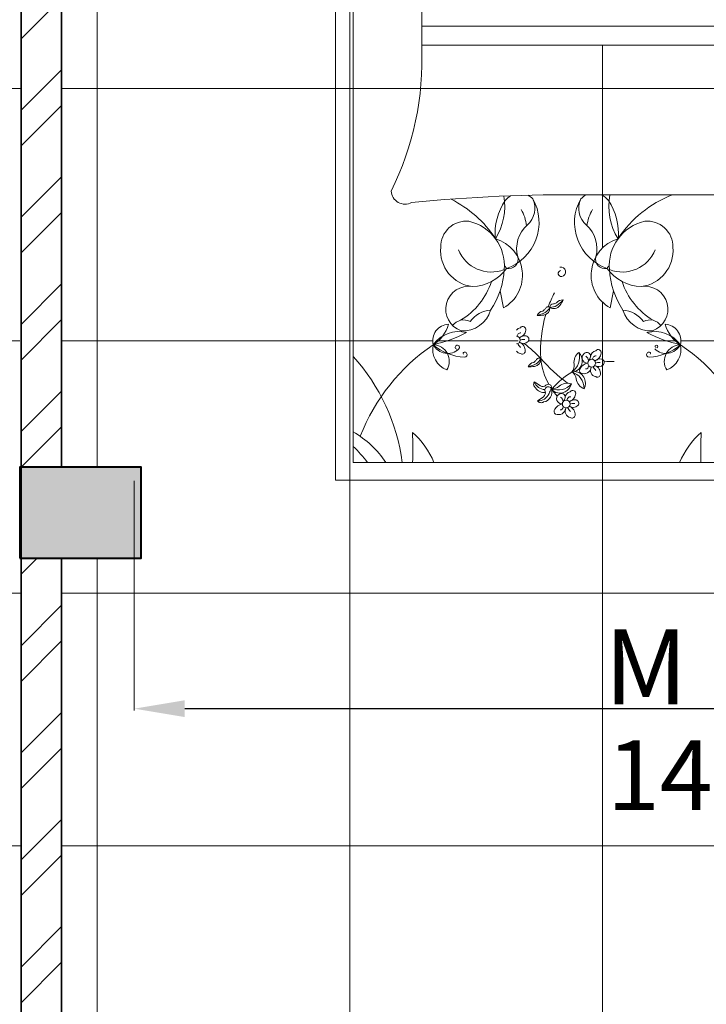
# Model space of a CAD drawing. Units: inches. Extents: x 351 to 1738, y -265 to 286.
# Tile 33 of 38: x 1380 to 1448, y 20 to 118. Entities that reach past the tile are written whole.
import ezdxf

# ---------------------------------------------------------------- set-up
doc = ezdxf.new("R2010")
doc.units = ezdxf.units.IN
doc.header["$MEASUREMENT"] = 0
for name, color, linetype, lineweight in [('A-ANNO-DIMS', 2, 'Continuous', 18), ('A-AREA-IDEN', 7, 'Continuous', 18), ('A-COLS', 7, 'Continuous', 40), ('A-COLS-PATT', 6, 'Continuous', 13), ('A-FLOR-PATT', 9, 'Continuous', 9), ('A-FURN', 18, 'Continuous', 13), ('A-WALL', 7, 'Continuous', 35), ('A-WALL-PATT', 152, 'Continuous', 13)]:
    doc.layers.add(name, color=color, linetype=linetype, lineweight=lineweight)
doc.styles.add('Annotative', font='arial.ttf')
doc.styles.get("Standard").update_dxf_attribs({"font": 'arial.ttf'})
doc.dimstyles.get("Standard").update_dxf_attribs({"dimtxt": 8, "dimasz": 5, "dimexe": 0.18, "dimexo": 0.0625, "dimgap": 0.09, "dimtad": 1, "dimtoh": 1, "dimzin": 0, "dimdsep": 46, "dimlunit": 4, "dimtxsty": 'Standard', "dimcen": 0, "dimclre": 256, "dimadec": 0, "dimazin": 0, "dimtfac": 1, "dimtofl": 0, "dimtmove": 0, "dimatfit": 3, "dimfxl": 1, "dimtolj": 1, "dimtzin": 0, "dimlwe": -1, "dimarcsym": 0})

# ---------------------------------------------------------------- blocks, each defined once
blk = doc.blocks.new('BED-DOUBLE-W-NIGHTSTANDS')
for p, q in [((121.406, 44.947), (28.441, 44.947)), ((121.549, 43.065), (28.441, 43.065)), ((106.084, 28.242), (44.816, 28.242)), ((36.536, 17.047), (36.202, 18.753)), ((47.082, 17.047), (47.416, 18.753))]:
    blk.add_line(p, q)
blk.add_lwpolyline([(28.513, 71.52, 0.001242), (28.441, 42.889, -0.127202), (25.416, 28.619)], format="xyb")
for points in [[(121.562, 54.359), (129.93, 54.359), (129.93, 0), (19.917, 0), (19.917, 54.359), (28.453, 54.359)], [(28.449, 52.61), (21.666, 52.61), (21.666, 1.749), (128.181, 1.749), (128.181, 52.61), (121.53, 52.61)]]:
    blk.add_lwpolyline(points)
for centre in [(45.254, 11.579), (42.74, 7.529)]:
    blk.add_circle(centre, 0.384)
for centre, radius, start, end in [((26.805, 28.716), 1.392, 183.97998, 297.34124), ((43.015, -128.837), 157.09, 89.34325, 95.68869), ((26.216, 17.616), 11.421, 33.66712, 63.29966), ((41.523, 24.412), 5.82, 145.78505, 184.73037), ((30.405, 27.126), 6.252, 328.82178, 9.15542), ((38.149, 26.573), 1.817, 120.0293, 142.32497), ((35.247, 25.502), 4.809, 289.28218, 29.1751), ((37.381, 26.933), 2.258, 311.56531, 23.83541), ((38.149, 26.573), 1.817, 44.45169, 63.55801), ((48.371, 25.502), 4.809, 150.8249, 250.71782), ((46.238, 26.933), 2.258, 156.16459, 228.43469), ((45.47, 26.573), 1.817, 113.22901, 135.54831), ((45.47, 26.573), 1.817, 37.67503, 66.71436), ((42.096, 24.412), 5.82, 355.26963, 34.21495), ((53.213, 27.126), 6.252, 169.71335, 211.17822), ((57.402, 17.616), 11.421, 111.49413, 146.33288), ((34.521, 24.631), 4.338, 7.43599, 29.91487), ((49.097, 24.631), 4.338, 150.08513, 172.56401), ((32.869, 23.1), 2.548, 84.48557, 181.05378), ((32.087, 21.215), 4.539, 355.29334, 76.921), ((51.531, 21.215), 4.539, 103.079, 184.70666), ((50.749, 23.1), 2.548, 358.94622, 95.51443), ((40.931, 22.929), 3.094, 131.56531, 195.14713), ((42.687, 22.929), 3.094, 344.85287, 48.43469), ((34.666, 20.299), 3.752, 299.90854, 73.1337), ((48.953, 20.299), 3.752, 106.8663, 240.09146), ((33.914, 22.735), 3.606, 174.94485, 262.88575), ((35.331, 24.102), 3.502, 201.58187, 291.42215), ((48.287, 24.102), 3.502, 248.57785, 338.41813), ((49.704, 22.735), 3.606, 277.11425, 5.05515), ((37.041, 21.876), 0.937, 257.30406, 15.14713), ((46.577, 21.876), 0.937, 164.85287, 282.69594), ((33.287, 23.537), 4.383, 272.3591, 324.04014), ((28.528, 21.336), 8.098, 326.28828, 356.5076), ((41.523, 24.412), 5.82, 212.70113, 216.34448), ((42.242, 20.456), 0.291, 102.70507, 280.43845), ((42.209, 20.635), 0.473, 280.43845, 100.41356), ((42.096, 24.412), 5.82, 323.65552, 327.29887), ((50.331, 23.537), 4.383, 215.95986, 267.6409), ((55.091, 21.336), 8.098, 183.4924, 213.71172), ((28.594, 21.91), 7.124, 301.26137, 341.7045), ((55.024, 21.91), 7.124, 198.2955, 238.73863), ((33.085, 16.925), 2.265, 80.26398, 250.86884), ((52.702, 12.86), 12.498, 153.0032, 159.89408), ((50.534, 16.925), 2.265, 289.13116, 99.73602), ((40.818, 19.778), 2.424, 285.51291, 293.60991), ((42.4, 17.052), 0.792, 87.35788, 140.49441), ((40.569, 19.327), 2.385, 301.16403, 321.56124), ((38.629, 19.743), 4.256, 324.68979, 333.49364), ((32.541, 17.606), 2.828, 265.96902, 344.3045), ((35.587, 13.847), 3.012, 96.1662, 141.58255), ((40.576, 15.96), 0.792, 101.32561, 154.46214), ((39.436, 18.648), 2.385, 280.25878, 300.65599), ((38.921, 18.642), 2.424, 308.21012, 316.30712), ((40.408, 17.049), 0.724, 278.34322, 4.28685), ((40.007, 17.685), 1.265, 300.65599, 332.63414), ((40.958, 16.849), 0.307, 55.76575, 157.44165), ((41.436, 17.136), 0.307, 84.37838, 186.05427), ((41.149, 18.368), 1.265, 269.18588, 301.16403), ((41.519, 17.714), 0.724, 237.53317, 323.47681), ((48.031, 13.847), 3.012, 38.41745, 83.8338), ((51.077, 17.606), 2.828, 195.6955, 274.03098), ((32.618, 14.471), 1.388, 63.97555, 143.26805), ((39.985, 20.555), 4.256, 268.32639, 277.13024), ((52.702, 12.86), 12.498, 163.58418, 183.82768), ((51, 14.471), 1.388, 36.73195, 116.02445), ((31.166, 13.794), 1.634, 92.95159, 193.72796), ((27.826, 16.28), 3.366, 301.38267, 345.29688), ((32.107, 11.586), 3.115, 75.46535, 144.23429), ((38.336, 14.458), 0.641, 101.56373, 142.6358), ((37.821, 14.961), 0.924, 288.72627, 352.50315), ((38.45, 14.916), 0.297, 345.23556, 144.9248), ((51.511, 11.586), 3.115, 35.76571, 104.53465), ((52.452, 13.794), 1.634, 346.27204, 87.04841), ((55.792, 16.28), 3.366, 194.70312, 238.61733), ((26.591, 26.864), 13.785, 282.51726, 297.18239), ((37.804, 13.863), 0.384, 273.27684, 86.72316), ((38.252, 14.227), 0.367, 91.10805, 181.86747), ((38.642, 13.489), 0.794, 80.3487, 133.65382), ((38.499, 14.146), 0.629, 229.78892, 317.67915), ((38.491, 12.663), 1.258, 83.08516, 105.71709), ((38.719, 13.945), 0.331, 317.67915, 80.3487), ((57.027, 26.864), 13.785, 242.81761, 257.48274), ((40.708, -2.855), 19.706, 124.38655, 158.59079), ((31.714, 12.942), 2.185, 167.71153, 249.03868), ((29.53, 11.762), 1.646, 328.46331, 88.28689), ((32.859, 17.159), 4.984, 228.84017, 267.9352), ((31.007, 14.156), 1.612, 207.6827, 313.77619), ((31.974, 13.146), 0.213, 313.77619, 249.71835), ((38.328, 13.152), 0.634, 217.76209, 259.04026), ((39.013, 13.997), 1.167, 203.42757, 227.61037), ((37.791, 12.814), 0.893, 355.05304, 68.36176), ((38.387, 12.763), 0.295, 232.47371, 355.05304), ((29.779, 2.226), 14.328, 43.15413, 52.0459), ((45.785, 12.175), 0.641, 101.56373, 176.36503), ((45.9, 12.632), 0.297, 345.23556, 144.9248), ((50.759, 17.159), 4.984, 272.0648, 311.15983), ((52.612, 14.156), 1.612, 226.22381, 332.3173), ((51.667, 13.227), 0.128, 290.26671, 226.22708), ((54.088, 11.762), 1.646, 91.71311, 211.53669), ((51.904, 12.942), 2.185, 290.96132, 12.28847), ((42.91, -2.855), 19.706, 21.40921, 55.61345), ((6.995, -0.907), 19.706, 7.74496, 41.8856), ((32.663, 12.546), 0.119, 101.4834, 217.94089), ((32.688, 12.423), 0.245, 267.9352, 101.4834), ((38.022, 13.564), 2.424, 308.21012, 316.30712), ((39.509, 11.972), 0.724, 278.34322, 4.28685), ((39.108, 12.607), 1.265, 300.65599, 332.63414), ((40.059, 11.772), 0.307, 55.76575, 157.44165), ((46.476, 12.545), 6.266, 184.75602, 209.20408), ((55.496, 25.887), 20.619, 222.24124, 232.17444), ((42.312, 12.15), 1.752, 304.53686, 16.36991), ((44.744, 11.659), 1.239, 127.31045, 187.92519), ((43.042, 11.798), 1.273, 355.01064, 41.65801), ((44.83, 12.114), 0.524, 126.10456, 271.42811), ((44.771, 12.256), 0.377, 353.75256, 131.70535), ((44.417, 11.809), 0.529, 0.06451, 61.15075), ((44.543, 12.26), 0.604, 311.84125, 355.78771), ((45.702, 11.943), 0.367, 91.10805, 181.86747), ((46.092, 11.205), 0.794, 80.3487, 133.65382), ((45.271, 12.677), 0.924, 288.72627, 352.50315), ((46.169, 11.661), 0.331, 317.67915, 80.3487), ((47.12, 4.223), 7.516, 87.10709, 94.75853), ((50.93, 12.423), 0.245, 78.5166, 272.0648), ((50.955, 12.546), 0.119, 322.05911, 78.5166), ((39.677, 10.882), 0.792, 101.32561, 154.46214), ((38.537, 13.571), 2.385, 280.25878, 300.65599), ((39.086, 15.478), 4.256, 268.32639, 277.13024), ((43.248, 11.759), 1.065, 272.84988, 356.12261), ((42.496, 11.346), 1.031, 321.76073, 7.92519), ((43.551, 9.683), 1.065, 20.5253, 88.5375), ((44.446, 10.858), 0.381, 148.0499, 225.62681), ((47.12, 4.223), 7.516, 113.05007, 113.84774), ((45.151, 10.418), 1.212, 104.75581, 148.0499), ((44.472, 11.286), 0.758, 247.40857, 351.43859), ((44.685, 11.255), 0.255, 262.90601, 7.13198), ((45.778, 10.868), 0.634, 151.21959, 259.04026), ((46.463, 11.713), 1.167, 203.42757, 227.61037), ((45.949, 11.862), 0.629, 229.78892, 317.67915), ((45.241, 10.53), 0.893, 355.05304, 68.36176), ((45.941, 10.379), 1.258, 83.08516, 105.71709), ((47.12, 4.223), 7.516, 120.54402, 139.81798), ((42.712, 9.864), 1.031, 8.72271, 54.88717), ((42.767, 9.04), 1.752, 0.278, 72.11105), ((44.956, 10.208), 1.239, 188.72271, 249.33746), ((43.365, 9.587), 1.273, 334.9899, 21.63727), ((45.837, 10.479), 0.295, 232.47371, 355.05304), ((39.944, 9.493), 0.429, 146.86359, 236.90213), ((45.994, 18.945), 11.227, 235.1882, 238.88441), ((40.68, 10.115), 1.162, 199.47987, 267.68284), ((40.551, 9.675), 1, 212.81548, 277.39917), ((40.422, 9.714), 0.444, 238.88441, 314.26458), ((40.325, 8.719), 1, 280.30568, 17.1958), ((40.241, 8.615), 0.444, 306.37461, 21.75478), ((40.965, 8.904), 0.335, 19.36054, 201.75478), ((40.966, 9.155), 0.335, 311.87034, 134.26458), ((47.267, 6.101), 6.693, 153.78194, 158.29129), ((41.94, 10.674), 1.752, 247.23048, 319.06353), ((41.362, 10.084), 1.031, 264.45436, 310.61881), ((46.476, 12.545), 6.266, 214.00334, 222.49171), ((42.116, 9.675), 1.065, 218.32082, 298.81623), ((42.84, 8.361), 1.239, 70.00407, 130.61881), ((42.038, 9.869), 1.273, 297.70426, 344.35163), ((43.386, 8.581), 0.297, 345.23556, 144.9248), ((39.969, 9.007), 1.162, 266.97007, 338.29129), ((33.846, 17.297), 11.227, 302.6784, 306.37461), ((40.262, 8.089), 0.429, 214.3538, 304.39233), ((42.316, 8.063), 0.524, 126.10456, 271.42811), ((42.258, 8.205), 0.377, 353.75256, 131.70535), ((41.904, 7.758), 0.529, 0.06451, 61.15075), ((42.029, 8.209), 0.604, 311.84125, 355.78771), ((43.272, 8.124), 0.641, 101.56373, 176.36503), ((43.188, 7.892), 0.367, 91.10805, 181.86747), ((43.578, 7.154), 0.794, 80.3487, 133.65382), ((42.757, 8.626), 0.924, 288.72627, 352.50315), ((43.656, 7.611), 0.331, 317.67915, 80.3487), ((41.933, 6.807), 0.381, 148.0499, 225.62681), ((42.638, 6.368), 1.212, 104.75581, 148.0499), ((41.958, 7.235), 0.758, 247.40857, 351.43859), ((42.171, 7.205), 0.255, 262.90601, 7.13198), ((43.264, 6.817), 0.634, 151.21959, 259.04026), ((43.949, 7.662), 1.167, 203.42757, 227.61037), ((43.436, 7.811), 0.629, 229.78892, 317.67915), ((42.727, 6.48), 0.893, 355.05304, 68.36176), ((43.427, 6.328), 1.258, 83.08516, 105.71709), ((43.323, 6.428), 0.295, 232.47371, 355.05304), ((16.881, -3.546), 9.602, 33.46172, 60.11157), ((22.259, -1.325), 8.012, 22.55474, 48.95456), ((0.311, 2.982), 27.264, 357.40811, 3.65191), ((61.36, -1.325), 8.012, 131.04544, 157.44526), ((83.307, 2.982), 27.264, 176.34809, 182.59189), ((13.426, -5.336), 11.966, 36.30357, 46.48142)]:
    blk.add_arc(centre, radius, start, end)
blk = doc.blocks.new('COL-9x12')
blk.add_lwpolyline([(0, 12), (0, 0), (9, 0), (9, 12)], close=True)
blk = doc.blocks.new('*D46')
at = {"layer": 'A-ANNO-DIMS', "transparency": 16777216}
for p, q in [((1391.393, 72.125), (1391.393, 49.373)), ((1542.294, 72.125), (1542.294, 49.373))]:
    blk.add_line(p, q, dxfattribs=at)
at = {"layer": 'A-ANNO-DIMS', "color": 0, "lineweight": -2, "transparency": 16777216}
for p, q in [((1396.393, 49.553), (1537.294, 49.553)), ((1542.294, 49.553), (1738.088, 49.553))]:
    blk.add_line(p, q, dxfattribs=at)
at = {"layer": 'A-ANNO-DIMS', "color": 0, "transparency": 16777216}
for points in [[(1396.393, 50.386), (1396.393, 48.72), (1391.393, 49.553)], [(1537.294, 50.386), (1537.294, 48.72), (1542.294, 49.553)]]:
    blk.add_solid(points, dxfattribs=at)
at = {"layer": 'Defpoints', "color": 0, "transparency": 16777216}
for p in [(1391.393, 72.188), (1542.294, 72.188), (1542.294, 49.553)]:
    blk.add_point(p, dxfattribs=at)
at = {"layer": 'A-ANNO-DIMS', "color": 0, "transparency": 16777216, "insert": (1642.691, 53.779), "char_height": 8, "attachment_point": 5}
blk.add_mtext('\\A1;BED AND NIGHTSTANDS 12\'-7" TYP.', dxfattribs=at)

msp = doc.modelspace()

# ---------------------------------------------------------------- hatches: boundary and pattern name
at = {"layer": 'A-COLS-PATT'}
h = msp.add_hatch(color=256, dxfattribs=at)
h.dxf.hatch_style = 1
h.paths.add_polyline_path([(1112.704, 237.963), (1103.704, 237.963), (1103.704, 228.963), (1112.704, 228.963)])
h.paths.add_polyline_path([(1115.704, 237.963), (1112.704, 237.963), (1112.704, 228.963), (1115.704, 228.963)])
h.paths.add_polyline_path([(1043.704, 255.963), (1034.704, 255.963), (1034.704, 243.963), (1043.704, 243.963)])
h.paths.add_polyline_path([(1043.704, 210.963), (1034.704, 210.963), (1034.704, 198.963), (1043.704, 198.963)])
h.paths.add_polyline_path([(1043.704, -45.037), (1034.704, -45.037), (1034.704, -57.037), (1043.704, -57.037)])
h.paths.add_polyline_path([(1112.704, -45.037), (1103.704, -45.037), (1103.704, -57.037), (1112.704, -57.037)])
h.paths.add_polyline_path([(1112.704, -161.037), (1103.704, -161.037), (1103.704, -164.037), (1103.704, -173.037), (1112.704, -173.037)])
h.paths.add_polyline_path([(1043.704, -161.037), (1034.704, -161.037), (1034.704, -173.037), (1043.704, -173.037)])
h.paths.add_polyline_path([(1248.549, -164.037), (1236.549, -164.037), (1236.549, -173.037), (1248.549, -173.037)])
h.paths.add_polyline_path([(1248.549, -50), (1236.549, -50), (1236.549, -59), (1248.549, -59)])
h.paths.add_polyline_path([(1248.704, 73.463), (1244.704, 73.463), (1244.704, 64.463), (1248.704, 64.463)])
h.paths.add_polyline_path([(1244.704, 73.463), (1236.704, 73.463), (1236.704, 64.463), (1244.704, 64.463)])
h.paths.add_polyline_path([(1248.704, 237.963), (1236.704, 237.963), (1236.704, 228.963), (1248.704, 228.963)])
h.paths.add_polyline_path([(1392.204, 237.963), (1380.204, 237.963), (1380.204, 228.963), (1392.204, 228.963)])
h.paths.add_polyline_path([(1536.064, 237.963), (1524.064, 237.963), (1524.064, 228.963), (1536.064, 228.963)])
h.paths.add_polyline_path([(1536.064, 73.463), (1524.064, 73.463), (1524.064, 64.463), (1536.064, 64.463)])
h.paths.add_polyline_path([(1384.204, 73.463), (1380.204, 73.463), (1380.204, 64.463), (1384.204, 64.463)])
h.paths.add_polyline_path([(1392.064, 73.463), (1384.204, 73.463), (1384.204, 64.463), (1392.064, 64.463)])
h.paths.add_polyline_path([(1536.064, -53.037), (1524.064, -53.037), (1524.064, -57.037), (1536.064, -57.037)])
h.paths.add_polyline_path([(1536.064, -48.037), (1524.064, -48.037), (1524.064, -53.037), (1536.064, -53.037)])
h.paths.add_polyline_path([(1392.064, -48.037), (1380.064, -48.037), (1380.064, -56.5), (1380.065, -57.037), (1392.064, -57.037)])
h.paths.add_polyline_path([(1536.064, -164.037), (1524.064, -164.037), (1524.064, -173.037), (1536.064, -173.037)])
at = {"layer": 'A-FLOR-PATT', "transparency": 33554559}
h = msp.add_hatch(dxfattribs=at)
h.set_pattern_fill('ANSI37', color=256, scale=200, angle=135)
h.set_pattern_definition([(180, (1112.704, -164.037), (-2e-15, -25), []), (270, (1112.704, -164.037), (25, -5e-15), [])])
h.paths.add_polyline_path([(1380.064, 73.463), (1380.132, 148.463), (1338.064, 148.463), (1290.704, 148.463), (1290.704, 88.463), (1248.704, 88.463), (1248.704, -2.009), (1244.704, -2.009), (1244.704, 142.457), (1160.704, 142.457), (1160.704, 158.963), (1160.704, 170.137), (1160.704, 206.137), (1160.704, 228.963), (1112.704, 228.963), (1112.704, 209.963), (1112.704, 168.963), (1124.704, 168.963), (1124.704, 162.963), (1112.704, 162.963), (1112.704, 64.463), (1112.704, 60.463), (1112.704, 0.463), (1112.704, -48.026), (1146.804, -47.981), (1146.804, -35.691), (1207.804, -35.691), (1207.804, -47.902), (1236.542, -47.864), (1236.544, -50.009), (1248.5, -50.009), (1248.506, -102.915), (1248.512, -150.915), (1248.514, -164.037), (1248.549, -164.037), (1273.017, -164.037), (1273.017, -128.799), (1355.24, -128.799), (1355.24, -164.037), (1384.204, -164.037), (1384.204, -57.037), (1380.064, -57.037), (1380.064, -48.037), (1392.064, -48.037), (1392.064, -53.037), (1406.549, -53.037), (1406.549, -57.037), (1401.204, -57.037), (1401.204, -147.037), (1468.204, -147.037), (1468.204, -138.5), (1472.204, -138.5), (1472.204, -102.5), (1468.204, -102.5), (1468.204, -57.037), (1442.549, -57.037), (1442.549, -53.037), (1463.049, -53.037), (1463.049, -40.747), (1524.049, -40.747), (1524.049, -48.037), (1536.064, -48.037), (1536.064, -53.037), (1557.704, -53.037), (1557.704, 204.963), (1384.204, 204.963), (1384.204, 73.463), (1392.064, 73.463), (1392.064, 64.463), (1384.204, 64.463), (1384.204, -3.5), (1380.204, -3.537), (1380.204, 64.463), (1380.064, 64.463)])
h.paths.add_polyline_path([(1510.714, 86.458, -0.103984), (1511.661, 85.595, 0.470438), (1510.158, 87.614, 0.0961)], flags=16)
h.paths.add_polyline_path([(1510.443, 100.266, 0.009798), (1504.693, 100.48, 0.02879), (1504.6, 99.767, -0.165331), (1505.519, 96.135, -0.143601)], flags=16)
h.paths.add_polyline_path([(1487.201, 85.595, -0.103984), (1488.148, 86.458, 0.0961), (1488.704, 87.614, 0.470438)], flags=0)
h.paths.add_polyline_path([(1495.052, 100.43), (1494.178, 100.43, -0.026463), (1494.262, 99.774, -0.144219)], flags=16)
h.paths.add_polyline_path([(1444.485, 86.458, -0.103984), (1445.433, 85.595, 0.470438), (1443.93, 87.614, 0.0961)], flags=16)
h.paths.add_polyline_path([(1420.972, 85.595, -0.103984), (1421.92, 86.458, 0.0961), (1422.475, 87.614, 0.470438)], flags=16)
h.paths.add_polyline_path([(1428.632, 100.335, 0.001054), (1427.971, 100.309, -0.021524), (1428.033, 99.774, -0.114301)], flags=16)
h.paths.add_polyline_path([(1419.906, 143.708, 0.024979), (1420.222, 157.526), (1421.573, 159.101), (1421.573, 175.369), (1391.393, 175.369), (1391.393, 200.519), (1542.294, 200.519), (1542.294, 175.369), (1512.028, 175.369, 0.019865), (1511.521, 153.838, 0.025134), (1512.758, 118.323, 0.020553), (1512.942, 115.253), (1419.834, 115.253, -0.000414), (1419.843, 124.798), (1413.059, 124.798), (1413.059, 84.437, -0.061853), (1415.831, 80.45, -0.093077), (1420.972, 85.595, -0.267537), (1422.371, 84.732, 0.08511), (1424.052, 84.616, -0.885393), (1424.033, 84.851, -1.125815), (1424.073, 84.366, -0.087987), (1422.371, 84.732, -0.267537), (1422.326, 83.089, -0.370542), (1420.972, 85.595, 0.093077), (1415.831, 80.45, -0.087414), (1417.914, 73.937), (1418.941, 73.937, 0.02725), (1418.913, 76.906, -0.115703), (1421.051, 73.937), (1445.354, 73.937, -0.115703), (1447.492, 76.906, 0.02725), (1447.464, 73.937), (1448.491, 73.937, -0.087414), (1450.574, 80.45, 0.093077), (1445.433, 85.595, -0.370542), (1444.079, 83.089, -0.267537), (1444.034, 84.732, -0.087987), (1442.332, 84.366, -1.125815), (1442.372, 84.851, -2.032736), (1442.364, 84.368, 0.086378), (1444.034, 84.732, -0.267537), (1445.433, 85.595, -0.093077), (1450.574, 80.45, -0.257732), (1466.483, 90.927, -0.47867), (1468.832, 91.907, -0.47867), (1471.18, 90.927, -0.26264), (1483.053, 81.78, -0.071866), (1487.201, 85.595, -0.267537), (1488.6, 84.732, 0.08511), (1490.28, 84.616, -0.885393), (1490.262, 84.851, -1.125815), (1490.301, 84.366, -0.087987), (1488.6, 84.732, -0.267537), (1488.554, 83.089, -0.370542), (1487.201, 85.595, 0.071866), (1483.053, 81.78, -0.132065), (1484.143, 73.937), (1485.169, 73.937, 0.02725), (1485.142, 76.906, -0.115703), (1487.28, 73.937), (1511.582, 73.937, -0.115703), (1513.72, 76.906, 0.02725), (1513.693, 73.937), (1514.719, 73.937, -0.087414), (1516.802, 80.45, 0.093077), (1511.661, 85.595, -0.370542), (1510.308, 83.089, -0.267537), (1510.262, 84.732, -0.087987), (1508.561, 84.366, -1.125815), (1508.601, 84.851, -2.032736), (1508.592, 84.368, 0.086378), (1510.262, 84.732, -0.267537), (1511.661, 85.595, -0.093077), (1516.802, 80.45, -0.061853), (1519.575, 84.437), (1519.575, 73.937), (1413.059, 73.937), (1413.059, 124.798), (1419.843, 124.798, -0.000821)], flags=16)
h.paths.add_polyline_path([(1220.149, 54.133, -0.103984), (1220.869, 53.476, 0.470438), (1219.727, 55.011, 0.0961)], flags=16)
h.paths.add_polyline_path([(1219.944, 64.626, 0.009798), (1215.574, 64.789, 0.02879), (1215.503, 64.247, -0.165331), (1216.201, 61.487, -0.143601)], flags=16)
h.paths.add_polyline_path([(1209.779, 64.449, 0.097446), (1209.339, 64.751), (1208.247, 64.751, 0.12739), (1207.7, 64.326, 0.171586), (1206.95, 61.475, -0.158854), (1207.636, 59.45, 0.015898), (1207.795, 59.218, 0.061546), (1208.598, 59.616, 0.175416), (1208.638, 60.099, -0.284779), (1209.348, 62.472, 0.326216)], flags=16)
h.paths.add_polyline_path([(1169.818, 54.133, -0.103984), (1170.538, 53.476, 0.470438), (1169.396, 55.011, 0.0961)], flags=16)
h.paths.add_polyline_path([(1159.017, 62.472, 0.284764), (1158.307, 60.099, -0.175433), (1158.267, 59.616, 0.39293), (1159.448, 64.449, -0.32623)], flags=16)
h.paths.add_polyline_path([(1156.342, 58.239, -0.178321), (1154.011, 55.31, -0.174736), (1154.722, 55.233, -0.200802), (1156.27, 56.086, 0.12699), (1157.283, 58.991, -0.091205)], flags=16)
h.paths.add_polyline_path([(1156.624, 61.413, 0.157275), (1157.316, 64.247, 0.169622)], flags=16)
h.paths.add_polyline_path([(1152.67, 54.133, -0.0961), (1151.95, 53.476, 0.064076), (1154.465, 54.384, 0.199016)], flags=16)
h.paths.add_polyline_path([(1202.281, 53.476, -0.103984), (1203, 54.133, 0.0961), (1203.423, 55.011, 0.470438)], flags=0)
h.paths.add_polyline_path([(1151.139, 97.64, 0.024979), (1151.379, 108.141), (1152.406, 109.338), (1152.406, 121.701), (1129.47, 121.701), (1129.47, 140.814), (1244.149, 140.814), (1244.149, 121.701), (1221.148, 121.701, 0.019865), (1220.763, 105.338, 0.025134), (1221.703, 78.349, 0.020553), (1221.843, 76.016), (1151.078, 76.016, -0.128743), (1148.786, 65.037, 0.539352), (1150.327, 64.171, -0.027594), (1163.481, 64.751, 0.097695), (1163.04, 64.449, 0.326216), (1163.471, 62.472, -0.284777), (1164.181, 60.099, -0.194757), (1165.846, 61.443, -0.155402), (1165.172, 64.247, -0.166022), (1165.869, 61.475, -0.177014), (1167.852, 62.77, -0.448203), (1169.974, 60.807, -0.393499), (1167.679, 57.86, -0.895548), (1168.438, 54.524, -0.355767), (1166.218, 56.086, -0.066024), (1165.505, 57.539), (1165.251, 56.243, -0.371732), (1164.02, 59.758, -0.373614), (1163.04, 64.449, -0.097695), (1163.481, 64.751, 0.021354), (1153.294, 64.429, -0.134183), (1156.695, 61.368, 0.186873), (1154.636, 62.77, 0.448203), (1152.514, 60.807, 0.403726), (1154.905, 57.846, 0.711219), (1153.334, 55, 0.53154), (1151.95, 53.476, -0.267537), (1153.013, 52.821, 0.08511), (1154.29, 52.732, -0.885393), (1154.276, 52.911, -1.125815), (1154.306, 52.543, -0.087987), (1153.013, 52.821, -0.267537), (1152.978, 51.572, -0.370542), (1151.95, 53.476, 0.093077), (1148.043, 49.566, -0.087414), (1149.626, 44.617), (1150.406, 44.617, 0.02725), (1150.385, 46.873, -0.115703), (1152.01, 44.617), (1170.478, 44.617, -0.115703), (1172.103, 46.873, 0.02725), (1172.082, 44.617), (1172.862, 44.617, -0.087414), (1174.445, 49.566, 0.093077), (1170.538, 53.476, -0.370542), (1169.51, 51.572, -0.267537), (1169.475, 52.821, -0.087987), (1168.182, 52.543, -1.125815), (1168.212, 52.911, -2.032736), (1168.206, 52.544, 0.086378), (1169.475, 52.821, -0.267537), (1170.538, 53.476, -0.093077), (1174.445, 49.566, -0.257732), (1186.536, 57.528, -0.47867), (1188.321, 58.273, -0.47867), (1190.106, 57.528, -0.26264), (1199.128, 50.577, -0.071866), (1202.281, 53.476, -0.267537), (1203.344, 52.821, 0.08511), (1204.621, 52.732, -0.885393), (1204.607, 52.911, -1.125815), (1204.637, 52.543, -0.087987), (1203.344, 52.821, -0.267537), (1203.309, 51.572, -0.370542), (1202.281, 53.476, 0.071866), (1199.128, 50.577, -0.132065), (1199.957, 44.617), (1200.737, 44.617, 0.02725), (1200.716, 46.873, -0.115703), (1202.341, 44.617), (1220.809, 44.617, -0.115703), (1222.434, 46.873, 0.02725), (1222.413, 44.617), (1223.193, 44.617, -0.087414), (1224.776, 49.566, 0.093077), (1220.869, 53.476, -0.370542), (1219.841, 51.572, -0.267537), (1219.806, 52.821, -0.087987), (1218.513, 52.543, -1.125815), (1218.543, 52.911, -2.032736), (1218.537, 52.544, 0.086378), (1219.806, 52.821, -0.267537), (1220.869, 53.476, -0.093077), (1224.776, 49.566, -0.061853), (1226.883, 52.597), (1226.883, 44.617), (1145.936, 44.617), (1145.936, 83.269), (1151.091, 83.269, -0.000821)], flags=16)
h.paths.add_polyline_path([(1218.01, 57.86, -0.895548), (1218.769, 54.524, -0.355767), (1216.549, 56.086, -0.066024), (1215.836, 57.539), (1215.582, 56.243, -0.371732), (1214.351, 59.758, -0.373614), (1213.371, 64.449, 0.326216), (1213.802, 62.472, -0.284777), (1214.512, 60.099, -0.194757), (1216.177, 61.443, -0.179991), (1218.183, 62.77, -0.448203), (1220.305, 60.807, -0.393499)], flags=16)
h.paths.add_polyline_path([(1424.735, 91.363, -0.393499), (1421.715, 95.241, -0.448203), (1424.507, 97.824, -0.179991), (1427.147, 96.077, -0.194757), (1429.338, 94.309, -0.284777), (1430.272, 97.432, 0.326216), (1430.839, 100.034, -0.373614), (1429.55, 93.861, -0.371732), (1427.929, 89.235), (1427.596, 90.941, -0.066024), (1426.657, 89.029, -0.355767), (1423.736, 86.973, -0.895548)], flags=16)
h.paths.add_polyline_path([(1238.033, 131.257, -1), (1227.329, 131.257, -1)], flags=0)
h.paths.add_polyline_path([(1235.357, 131.257, -1), (1230.005, 131.257, -1)], flags=0)
h.paths.add_polyline_path([(1214.039, 54.243, 0.154382), (1214.38, 53.992, 0.358955), (1213.613, 54.016, 0.603948), (1214.379, 53.657, 0.371319), (1213.968, 52.872, 0.187994), (1214.312, 52.809, -0.592455), (1213.953, 52.967, -0.294279), (1214.083, 53.691, -1.300187), (1213.881, 54.134, -0.283762), (1214.469, 53.896, 1.15094)], flags=16)
h.paths.add_polyline_path([(1212.091, 56.286, -0.408434), (1211.337, 56.445, -0.036259), (1211.098, 56.848, -0.236098), (1211.59, 56.63, 0.035345), (1211.835, 56.543, -0.475241), (1212.091, 56.286, -0.475241), (1212.438, 56.182, 0.035345), (1212.631, 56.007, -0.236098), (1213.056, 55.676, -0.036259), (1212.588, 55.697, -0.408434)], flags=16)
h.paths.add_polyline_path([(1211.469, 50.297, 0.296043), (1210.47, 50.527, 0.310883), (1211.931, 50.148, 0.021255)], flags=16)
h.paths.add_polyline_path([(1213.739, 51.818, -0.036259), (1213.271, 51.838, -0.408434), (1212.774, 52.427, -0.094786), (1212.293, 50.703, 1.150474), (1212.911, 50.232, 0.166288), (1213.265, 50.68, -0.025254), (1212.603, 50.13, 1.087932), (1212.471, 49.407, 0.166288), (1213.02, 49.251, -0.016128), (1212.567, 49.563, -0.286859), (1212.217, 49.638, 0.022156), (1212.046, 50.055, -0.64613), (1212.185, 50.498, 0.088412), (1212.732, 52.077, -1.186037), (1213.121, 52.323, 0.035345), (1213.314, 52.148, -0.236098)], flags=16)
h.paths.add_polyline_path([(1212.094, 50.342, -0.048524), (1211.54, 49.605, -1.103834), (1211.397, 48.738, -0.785515), (1211.683, 48.254, -0.392043), (1210.948, 48.525, -0.392819), (1210.561, 47.995, -0.592455), (1210.201, 48.153, -0.294279), (1210.331, 48.877, -0.704172), (1210.316, 49.592, -0.679344), (1210.729, 50.112, 0.563676)], flags=16)
h.paths.add_polyline_path([(1211.274, 49.829, -0.139826), (1210.745, 49.859, -0.217879), (1210.948, 49.509, -0.498572)], flags=0)
h.paths.add_polyline_path([(1433.426, 81.49, -0.181571), (1434.245, 81.788, -0.008067), (1433.726, 82.205, 0.045578), (1432.755, 81.242, 0.179011)], flags=16)
h.paths.add_polyline_path([(1434.146, 81.009, -0.132442), (1433.645, 80.771, 0.259089), (1433.234, 80.471, -0.180211), (1433.392, 80.805, -0.16994), (1432.758, 81.109, 0.032652), (1433.273, 80.474, -0.493363), (1434.046, 80.146, -0.390497)], flags=16)
h.paths.add_polyline_path([(1434.83, 80.047, -0.947538), (1435.294, 79.576, -0.299128), (1434.625, 79.404, -0.270439), (1435.01, 78.591, -0.592455), (1434.537, 78.382, -0.392819), (1434.027, 79.08, -0.392043), (1433.06, 78.723, -0.352042), (1433.003, 79.197, -0.197216), (1433.75, 79.734, -0.71364), (1434.447, 79.939, -0.21479), (1434.819, 80.475, 0.408833), (1435.075, 80.803, -0.226152)], flags=16)
h.paths.add_polyline_path([(1432.67, 81.217, -0.454218), (1431.897, 79.923, -0.414411), (1431.301, 80.035, 0.016129), (1431.897, 80.445, 0.27957), (1432.073, 80.871, -0.289504), (1431.103, 81.321, -0.414411), (1430.978, 81.915, 0.01613), (1431.586, 81.521, 0.341293), (1432.125, 81.583, -0.813186)], flags=16)
h.paths.add_polyline_path([(1429.893, 86.381, -0.947538), (1430.358, 85.91, -0.173106), (1429.984, 85.712, -0.038817), (1431.625, 84.214, -0.0879), (1432.097, 88.549, -0.049768), (1431.254, 88.49, -0.236098), (1431.814, 88.925, 0.035345), (1432.067, 89.155, -0.475241), (1432.524, 89.291, -0.475241), (1432.86, 89.63, 0.035345), (1433.182, 89.744, -0.236098), (1433.83, 90.032, -0.036259), (1433.516, 89.502, -0.408434), (1432.524, 89.291, -0.312424), (1432.106, 88.58, 0.088559), (1431.625, 84.214, -0.408434), (1430.971, 83.439, -0.036259), (1430.355, 83.412, -0.236098), (1430.914, 83.847, 0.035345), (1431.168, 84.078, -0.475241), (1431.625, 84.214, 0.038817), (1429.984, 85.712, -0.321732), (1429.333, 86.048, -0.32743), (1429.883, 86.809, 0.408833), (1430.138, 87.138, -0.226152)], flags=16)
h.paths.add_polyline_path([(1211.206, 58.616, -0.999784), (1211.336, 59.323, -0.614994)], flags=16)
h.paths.add_polyline_path([(1210.288, 49.429, 0.154382), (1210.629, 49.178, 0.358955), (1209.861, 49.202, 0.603948), (1210.627, 48.843, -0.534825), (1210.806, 49.295, 0.748346)], flags=16)
h.paths.add_polyline_path([(1209.589, 51.828, -0.008791), (1209.775, 51.753, 0.112231), (1209.466, 52.019, 1.418851), (1209.014, 51.708, -0.458726), (1208.651, 51.073, -0.592455), (1208.291, 51.232, -0.294279), (1208.421, 51.955, -1.300187), (1208.219, 52.398, -0.226005), (1208.719, 52.257, -0.475519), (1209.158, 52.369, -1.455499), (1209.603, 52.664, 0.421305), (1209.191, 52.262, -0.591212), (1208.979, 51.796, 0.497399), (1209.773, 51.333, 0.649312)], flags=16)
h.paths.add_polyline_path([(1208.029, 52.041, 0.544667), (1208.832, 52.045, 0.220132)], flags=0)
h.paths.add_polyline_path([(1210.438, 51.425, -0.2042), (1210.277, 52.018, 0.270826), (1209.915, 52.897, 0.324115)], flags=0)
h.paths.add_polyline_path([(1209.668, 52.407, -0.60139), (1208.99, 52.221, -0.394916), (1208.248, 52.83, -0.836792), (1208.651, 53.017, -0.338488), (1209.039, 52.571, 0.194138), (1209.191, 52.262, 0.413995), (1209.712, 52.475, 0.51771), (1210.503, 51.416, 0.401922), (1209.493, 50.93, 0.206396), (1209.516, 50.165, -0.319463), (1210.417, 51.418, -0.466635)], flags=16)
h.paths.add_polyline_path([(1206.601, 56.086, -0.355767), (1204.381, 54.524, -0.921198), (1205.236, 57.846, 0.206569), (1207.614, 58.991, -0.12699)], flags=16)
h.paths.add_polyline_path([(1435.487, 82.816, 0.527765), (1436.615, 83.361, 0.50854), (1437.05, 82.433, 0.592455), (1437.524, 82.641, 0.331245), (1436.963, 83.548, 0.387863), (1437.808, 83.626, 0.592954), (1437.618, 84.176, 0.226016), (1436.961, 83.99, 0.318205), (1437.588, 84.854, 0.689374), (1437.05, 84.991, 0.335765), (1436.539, 84.41, -0.156993), (1436.404, 84.065, -0.434611), (1436.961, 83.99, -0.21479), (1437.333, 84.526, 0.408833), (1437.588, 84.854, -0.226152), (1437.343, 84.097, -0.947538), (1437.808, 83.626, -0.299128), (1437.139, 83.455, -0.270439), (1437.524, 82.641, -0.592455), (1437.05, 82.433, -0.392819), (1436.541, 83.13, -0.43966), (1435.475, 82.794, -0.174614), (1435.942, 82.244, -0.206396), (1435.912, 81.237, -0.270826), (1435.125, 82.208, 0.207976), (1434.686, 82.904, -0.196495)], flags=16)
h.paths.add_polyline_path([(1435.386, 84.832, 0.270811), (1434.91, 83.676, -0.204217), (1434.699, 82.895, 0.324115)], flags=0)
h.paths.add_polyline_path([(1435.68, 84.18, -0.217656), (1435.554, 83.304, -0.176705), (1436.236, 83.778, -0.373036)], flags=0)
h.paths.add_polyline_path([(1435.566, 100.034, 0.326216), (1436.133, 97.432, -0.284777), (1437.067, 94.309, -0.194757), (1439.258, 96.077, -0.155402), (1438.371, 99.767, -0.166022), (1439.289, 96.12, -0.177014), (1441.897, 97.824, -0.448203), (1444.69, 95.241, -0.393499), (1441.67, 91.363, -0.895548), (1442.669, 86.973, -0.355767), (1439.748, 89.029, -0.066024), (1438.809, 90.941), (1438.476, 89.235, -0.371732), (1436.855, 93.861, -0.373614)], flags=16)
h.paths.add_polyline_path([(1191.252, 49.507, -0.274022), (1190.658, 48.409, 0.267537), (1191.311, 47.344, 0.370542)], flags=0)
h.paths.add_polyline_path([(1190.301, 49.717, 0.199016), (1188.619, 49.04, 0.064076), (1191.252, 49.507, -0.0961)], flags=0)
h.paths.add_polyline_path([(1189.518, 47.857, 1.125815), (1189.676, 47.523, 2.044605)], flags=0)
h.paths.add_polyline_path([(1464.974, 80.372, 0.274022), (1465.756, 78.927, -0.083013)], flags=0)
h.paths.add_polyline_path([(1464.974, 80.372, 0.370542), (1464.897, 77.525, 0.576324)], flags=0)
h.paths.add_polyline_path([(1464.974, 80.372, -0.470438), (1467.284, 81.372, -0.0961), (1466.226, 80.648, -0.199016), (1468.439, 79.757, -0.064076)], flags=0)
h.paths.add_polyline_path([(1189.511, 56.43, -0.259467), (1188.321, 56.391, -0.259467), (1187.13, 56.43, 0.08511), (1188.193, 55.716, -0.885393), (1188.27, 55.878, -1.196013), (1188.355, 55.442, 0.101459)], flags=0)
h.paths.add_polyline_path([(1188.321, 57.596, 0.078072), (1187.678, 57.24, 0.01555), (1188.321, 57.136, 0.01555), (1188.964, 57.24, 0.078072)], flags=0)
h.paths.add_polyline_path([(1190.164, 55.365, -0.576324), (1190.106, 57.528, -0.198294), (1188.321, 58.319, -0.198294), (1186.536, 57.528, -0.576324), (1186.477, 55.365, -0.370542), (1186.536, 57.528, 0.198294), (1188.321, 58.319, 0.198294), (1190.106, 57.528, -0.370542)], flags=0)
h.paths.add_polyline_path([(1188.372, 55.878, 1.125814), (1188.529, 55.544, 2.044605)], flags=0)
h.paths.add_polyline_path([(1186.341, 49.717, -0.0961), (1185.389, 49.507, 0.064076), (1188.022, 49.04, 0.199016)], flags=0)
h.paths.add_polyline_path([(1185.389, 49.507, -0.267537), (1185.984, 48.409, 0.08511), (1187.046, 47.695, -0.885393), (1187.123, 47.857, -1.125815), (1186.966, 47.523, -0.087987), (1185.984, 48.409, -0.267537), (1185.331, 47.344, -0.370542)], flags=0)
h.paths.add_polyline_path([(1399.441, 187.944, -1), (1413.525, 187.944, -1)], flags=0)
h.paths.add_polyline_path([(1402.962, 187.944, -1), (1410.004, 187.944, -1)], flags=0)
h.paths.add_polyline_path([(1357.663, -72.245), (1377.272, -72.245), (1377.272, -91.854), (1357.663, -91.854)], flags=16)
h.paths.add_polyline_path([(1467.256, 78.201, -1.125815), (1467.049, 77.761, -2.044605)], flags=0)
h.paths.add_polyline_path([(1468.822, 88.714, 0.941125), (1469.106, 88.316, 1.137152), (1468.765, 88.755, 0.890986), (1468.99, 88.245, 0.094828), (1470.398, 89.481, -0.267537), (1471.18, 90.927, -0.028123), (1469.678, 90.547, -0.028774), (1469.948, 90.311, -0.020327), (1468.832, 90.41, -0.020327), (1467.716, 90.311, -0.028774), (1467.986, 90.547, -0.028123), (1466.483, 90.927, -0.267537), (1467.265, 89.481, 0.08511), (1468.663, 88.542, -1.202316)], flags=0)
h.paths.add_polyline_path([(1178.25, 124.523, -0.119929), (1165.65, 124.145, -0.107349), (1159.133, 124.446, -0.102891), (1159.132, 130.465, -0.074897), (1158.993, 137.956, 0.002027), (1167.844, 137.479, -0.07553), (1180.337, 137.666, -0.075861), (1186.502, 137.688, -0.14099), (1186.272, 130.046, -0.095481), (1186.729, 124.748, -0.10603)], flags=0)
h.paths.add_polyline_path([(1469.225, 79.757, -0.199016), (1471.437, 80.648, -0.0961), (1470.379, 81.372, -0.470438), (1472.689, 80.372, -0.370542), (1472.766, 77.525, -0.267537), (1471.907, 78.927, -0.087986), (1470.615, 77.761, -1.125849), (1470.408, 78.201, -2.032736), (1470.642, 77.778, 0.086378), (1471.907, 78.927, -0.267537), (1472.689, 80.372, -0.064076)], flags=0)
h.paths.add_polyline_path([(1430.423, 186.902, -0.074897), (1430.24, 196.758, 0.002027), (1441.887, 196.131, -0.07553), (1458.326, 196.377, -0.075861), (1466.438, 196.406, -0.14099), (1466.136, 186.35, -0.095481), (1466.737, 179.378, -0.10603), (1455.58, 179.082, -0.119929), (1439, 178.585, -0.107349), (1430.425, 178.981, -0.102891)], flags=0)
h.paths.add_polyline_path([(1162.258, 49.939, 0.335765), (1161.87, 49.497, -0.156994), (1161.767, 49.235, -0.434611), (1162.19, 49.178, -0.21479), (1162.473, 49.585, 1.529195)], flags=16)
h.paths.add_polyline_path([(1161.683, 49.021, 0.581518), (1161.268, 49.583, 0.592761)], flags=16)
h.paths.add_polyline_path([(1162.602, 48.058, 0.371319), (1162.192, 48.843, 0.434533), (1162.88, 48.962, 0.185081), (1162.197, 48.926, 1.121837)], flags=16)
h.paths.add_polyline_path([(1161.443, 48.941, -1.307104), (1161.495, 48.571, -0.217752), (1161.136, 48.254, 0.697303), (1161.871, 49.048, 0.121514)], flags=16)
h.paths.add_polyline_path([(1162.531, 49.429, -0.207084), (1162.05, 49.146, -0.99203)], flags=16)
h.paths.add_polyline_path([(1161.304, 49.578, -0.719667), (1161.513, 50.079, -0.130428), (1160.836, 50.168, 0.039593)], flags=0)
h.paths.add_polyline_path([(1162.036, 50.584, -0.008067), (1161.642, 50.9, 0.029367), (1161.35, 50.297, -0.205788)], flags=16)
h.paths.add_polyline_path([(1162.882, 51.392, -0.124733), (1162.763, 51.828, -0.101191), (1162.399, 51.438, -0.153425)], flags=0)
h.paths.add_polyline_path([(1164.235, 51.85, -0.309107), (1164.513, 51.136, -0.627125), (1163.781, 51.603, -0.685909), (1162.777, 51.219, -0.233285), (1163.303, 50.165, -0.270826), (1162.705, 50.903, 0.2042), (1162.381, 51.425, 0.204182), (1162.542, 52.018, -0.270841), (1162.903, 52.897, -0.127261), (1163.219, 52.529, -1.168681), (1163.781, 52.587, -0.329112), (1164.168, 53.017, -0.836792), (1164.571, 52.83, -0.193341), (1164.391, 52.338, -0.947538), (1164.744, 51.981, -0.299128)], flags=16)
h.paths.add_polyline_path([(1163.598, 51.937, -1.262956), (1163.236, 51.831, 0.012575), (1162.971, 51.721, 0.230657), (1163.151, 52.407, -0.164898), (1163.178, 52.661, -0.44932), (1163.628, 52.262, -0.721477), (1164.154, 52.088, -0.849998)], flags=0)
h.paths.add_polyline_path([(1161.613, 58.616, -0.980413), (1161.525, 59.049, -2.908935)], flags=16)
h.paths.add_polyline_path([(1160.252, 49.166, -0.414411), (1159.799, 49.251, 0.016129), (1160.252, 49.563, 0.27957), (1160.386, 49.887, -0.289504), (1159.649, 50.229, -0.414411), (1159.554, 50.68, 0.01613), (1160.015, 50.381, 0.617885), (1160.526, 50.703, -0.094786), (1160.045, 52.427, -0.140444), (1159.682, 52.042, -0.057856), (1159.3, 51.872, 0.544843), (1160.046, 52.419, -0.088122), (1160.404, 55.721, -0.049768), (1159.763, 55.676, -0.236098), (1160.188, 56.007, 0.035345), (1160.381, 56.182, -0.475241), (1160.728, 56.286, -0.475241), (1160.984, 56.543, 0.035345), (1161.229, 56.63, -0.236098), (1161.721, 56.848, -0.036259), (1161.482, 56.445, -0.408434), (1160.728, 56.286, -0.312424), (1160.411, 55.745, 0.088559), (1160.045, 52.427, 0.107081), (1160.634, 50.498, -0.494798), (1160.839, 50.149, -0.454218)], flags=16)
h.paths.add_polyline_path([(1160.666, 49.808, -2.076528), (1160.828, 50.172, 0.019586)], flags=0)
h.paths.add_polyline_path([(1158.439, 53.992, 0.154382), (1158.78, 54.243, 0.748346), (1158.262, 54.109, -0.338225), (1158.492, 53.839, -0.170816), (1159.124, 53.779, 0.495729), (1158.938, 54.134, 0.226016)], flags=16)
h.paths.add_polyline_path([(1160.045, 52.427, 0.038817), (1158.798, 53.565, -0.119818), (1158.574, 53.586, -0.309107), (1158.851, 52.872, -0.187994), (1158.506, 52.809, 0.592455), (1158.866, 52.967, 0.331245), (1158.44, 53.657, 0.201245), (1158.798, 53.565, -0.034023), (1159.901, 52.578, -0.044253), (1159.698, 52.323, -0.475241)], flags=16)
h.paths.add_polyline_path([(1336.926, -95.392), (1336.926, -117.945), (1291.82, -117.945), (1291.82, -95.392)], flags=16)
h.paths.add_polyline_path([(1357.535, -97.244), (1357.726, -96.697, 0.034844)], flags=16)
h.paths.add_polyline_path([(1376.693, -96.478), (1377.301, -96.5, 0.031497), (1375.907, -96.424), (1357.726, -96.424)], flags=16)
h.paths.add_polyline_path([(1379.403, -119.667, 0.026706), (1380.043, -119.439, -0.015299)], flags=16)
h.paths.add_polyline_path([(1357.726, -120.202), (1357.821, -120.202), (1357.821, -120.201)], flags=16)
h.paths.add_polyline_path([(1354.171, -104.592), (1354.469, -98.672, 0.011138)], flags=16)
h.paths.add_polyline_path([(1355.058, -119.136), (1354.578, -118.539, 0.143164)], flags=16)
h.paths.add_polyline_path([(1378.851, -96.821), (1378.85, -96.82), (1378.85, -96.82, -0.04968), (1380.055, -97.191), (1378.85, -96.82, 0.150054), (1375.135, -97.188), (1375.136, -119.44, -0.00997), (1374.747, -116.649), (1357.726, -116.649, 0.169385), (1357.535, -119.382), (1357.535, -119.382), (1357.535, -119.382, 0.034818), (1357.726, -119.928), (1357.726, -119.928), (1357.726, -119.929, -0.034877), (1357.535, -119.382), (1355.507, -119.382), (1355.317, -119.278), (1357.535, -119.382, -0.169394), (1357.726, -116.649, -0.039151), (1374.686, -116.113, -0.002015), (1374.625, -115.546, 0.115322), (1369.915, -115.474, 0.060921), (1369.922, -101.154, 0.115146), (1374.625, -101.079, -0.002016), (1374.686, -100.513, -0.039151), (1357.726, -99.977), (1374.747, -99.977, -0.009963), (1375.135, -97.188), (1375.135, -97.188, -0.150108)], flags=16)
h.paths.add_polyline_path([(1490.963, 91.363, -0.393499), (1487.944, 95.241, -0.448203), (1490.736, 97.824, -0.179991), (1493.376, 96.077, -0.194757), (1495.567, 94.309, -0.284777), (1496.501, 97.432, 0.326216), (1497.068, 100.034, -0.373614), (1495.778, 93.861, -0.371732), (1494.158, 89.235), (1493.824, 90.941, -0.066024), (1492.886, 89.029, -0.355767), (1489.964, 86.973, -0.895548)], flags=16)
h.paths.add_polyline_path([(1354.86, -97.658), (1355.316, -97.348, 0.101911)], flags=16)
h.paths.add_polyline_path([(1497.063, 83.327, 0.176724), (1496.37, 83.785, -0.405139), (1496.016, 83.384, 0.497399), (1497.06, 82.774, 0.649312), (1496.818, 83.426, -0.008791)], flags=16)
h.paths.add_polyline_path([(1496.339, 83.783, 0.592761), (1496.886, 84.522, 0.581518)], flags=16)
h.paths.add_polyline_path([(1495.11, 82.641, 0.592455), (1495.583, 82.433, 0.676915), (1495.805, 83.59, 0.375669)], flags=16)
h.paths.add_polyline_path([(1495.015, 84.176, -0.145057), (1495.301, 84.526, -0.408833), (1495.045, 84.854, 0.220629), (1495.381, 84.152, -0.199594), (1495.851, 83.764, -0.524017), (1494.826, 83.626, -0.592998)], flags=16)
h.paths.add_polyline_path([(1501.655, 81.915, -0.016129), (1501.048, 81.521, -0.392719), (1500.462, 81.37, -0.21067), (1500.607, 81.142, 0.306699)], flags=16)
h.paths.add_polyline_path([(1500.11, 89.291, -0.408434), (1499.118, 89.502, -0.036259), (1498.803, 90.032, -0.236098), (1499.451, 89.744, 0.035345), (1499.774, 89.63, -0.475241), (1500.11, 89.291, -0.475241), (1500.567, 89.155, 0.035345), (1500.82, 88.925, -0.236098), (1501.379, 88.49, -0.036259), (1500.763, 88.516, -0.408434)], flags=16)
h.paths.add_polyline_path([(1498.908, 82.205, -0.051322), (1500.013, 81.134, -0.587931), (1500.234, 81.676, 0.107081), (1501.009, 84.214, -0.03529)], flags=16)
h.paths.add_polyline_path([(1496.93, 83.875, -0.206396), (1497.247, 84.832, -0.270826), (1497.724, 83.676, 0.207976), (1497.944, 82.884, -0.381455)], flags=16)
h.paths.add_polyline_path([(1496.721, 81.237, 0.270812), (1497.509, 82.208, -0.204216), (1497.935, 82.895, 0.324115)], flags=16)
h.paths.add_polyline_path([(1497.529, 80.125, -0.145057), (1497.814, 80.475, -0.703182), (1498.282, 81.178, -0.122925), (1497.977, 81.714, -0.270837), (1499.207, 81.49, 0.207964), (1499.993, 81.248, -0.265145), (1499.278, 80.472, 0.381901), (1498.808, 79.947, -0.305905), (1498.848, 79.519, 0.499482), (1498.574, 79.217, -0.458726), (1498.097, 78.382, -0.592455), (1497.624, 78.591, -0.270439), (1498.009, 79.404, -0.299116), (1497.34, 79.576, -0.593016)], flags=16)
h.paths.add_polyline_path([(1500.736, 79.923, 0.414411), (1501.333, 80.035, -0.321648), (1500.192, 80.765, 0.019886), (1499.976, 81.251, 0.465331)], flags=16)
h.paths.add_polyline_path([(1501.009, 84.214, -0.038817), (1502.649, 85.712, -0.173095), (1502.276, 85.91, -0.593016), (1502.465, 86.46, -0.145057), (1502.751, 86.809, -0.408833), (1502.495, 87.138, 0.220629), (1502.831, 86.436, -0.199594), (1503.301, 86.048, -0.321732), (1502.649, 85.712, 0.038817), (1501.009, 84.214, 0.122449), (1501.412, 83.755, 0.475491), (1501.335, 84.226, 0.055822), (1501.719, 83.847, -0.236098), (1502.278, 83.412, -0.036259), (1501.663, 83.439, -0.408434)], flags=16)
h.paths.add_polyline_path([(1501.794, 100.034, 0.326216), (1502.362, 97.432, -0.284777), (1503.295, 94.309, -0.194757), (1505.486, 96.077, -0.179991), (1508.126, 97.824, -0.448203), (1510.918, 95.241, -0.393499), (1507.899, 91.363, -0.895548), (1508.898, 86.973, -0.355767), (1505.976, 89.029, -0.066024), (1505.038, 90.941), (1504.704, 89.235, -0.371732), (1503.084, 93.861, -0.373614)], flags=16)
h.paths.add_polyline_path([(1146.29, 131.257, -1), (1135.587, 131.257, -1)], flags=0)
h.paths.add_polyline_path([(1143.614, 131.257, -1), (1138.262, 131.257, -1)], flags=0)
h.paths.add_polyline_path([(1524.064, 73.463), (1536.064, 73.463), (1536.064, 64.463), (1524.064, 64.463)], flags=16)
h.paths.add_polyline_path([(1520.162, 187.944, -1), (1534.246, 187.944, -1)], flags=0)
h.paths.add_polyline_path([(1530.725, 187.944), (1527.204, 187.944), (1527.204, 184.423, 0.414214)], flags=0)
h.paths.add_polyline_path([(1278.415, -91.154), (1331.067, -91.154), (1331.067, -80.583), (1278.415, -80.583)], flags=24)
h.paths.add_polyline_path([(1266.655, -79.354), (1354.738, -79.354), (1354.738, -67.817), (1266.655, -67.817)], flags=24)
h.paths.add_polyline_path([(1115.482, 206.184), (1155.098, 206.184), (1155.098, 217.714), (1115.482, 217.714)], flags=24)
h.paths.add_polyline_path([(1161.771, 8.501), (1222.466, 8.501), (1222.466, 19.079), (1161.771, 19.079)], flags=24)
h.paths.add_polyline_path([(1164.656, 18.795), (1210.615, 18.795), (1210.615, 30.324), (1164.656, 30.324)], flags=24)
h.paths.add_polyline_path([(1368.147, -32.882), (1379.362, -32.882), (1379.362, -21.733), (1368.147, -21.733)], flags=24)
h.paths.add_polyline_path([(1244.842, -31.012), (1256.057, -31.012), (1256.057, -19.863), (1244.842, -19.863)], flags=24)
h.paths.add_polyline_path([(1114.589, 195.739), (1156.517, 195.739), (1156.517, 206.31), (1114.589, 206.31)], flags=24)
h.paths.add_polyline_path([(1436.398, 37.632), (1505.131, 37.632), (1505.131, 48.203), (1436.398, 48.203)], flags=24)
h.paths.add_polyline_path([(1435.991, 47.919), (1507.906, 47.919), (1507.906, 59.456), (1435.991, 59.456)], flags=24)
h.paths.add_polyline_path([(1415.107, -124.896), (1457.038, -124.896), (1457.038, -114.318), (1415.107, -114.318)], flags=24)
h.paths.add_polyline_path([(1417.992, -114.602), (1457.609, -114.602), (1457.609, -103.073), (1417.992, -103.073)], flags=24)
at = {"layer": 'A-WALL-PATT'}
h = msp.add_hatch(dxfattribs=at)
h.set_pattern_fill('ANSI32', color=256, scale=20)
h.set_pattern_definition([(45, (1034.704, -173.037), (-5.3033, 5.3033), []), (45, (1038.24, -173.037), (-5.3033, 5.3033), [])])
h.paths.add_polyline_path([(1043.704, -57.037), (1034.704, -57.037), (1034.704, -81.037), (1043.704, -81.037)])
h.paths.add_polyline_path([(1043.704, 198.963), (1034.704, 198.963), (1034.704, -45.037), (1043.704, -45.037)])
h.paths.add_polyline_path([(1043.704, 243.963), (1034.704, 243.963), (1034.704, 237.963), (1034.704, 210.963), (1043.704, 210.963)])
h.paths.add_polyline_path([(1112.704, 255.963), (1043.704, 255.963), (1043.704, 246.963), (1103.704, 246.963), (1103.704, 237.963), (1112.704, 237.963), (1112.704, 251.963)])
h.paths.add_polyline_path([(1056.704, 207.963), (1043.704, 207.963), (1043.704, 198.963), (1056.704, 198.963)])
h.paths.add_polyline_path([(1103.704, 207.963), (1092.704, 207.963), (1092.704, 198.963), (1103.704, 198.963)])
h.paths.add_polyline_path([(1112.704, 228.963), (1103.704, 228.963), (1103.704, 74.963), (1112.704, 74.963), (1112.704, 97.5)])
h.paths.add_polyline_path([(1284.129, -164.037), (1248.549, -164.037), (1248.549, -173.037), (1284.129, -173.037)])
h.paths.add_polyline_path([(1524.064, -164.037), (1472.204, -164.037), (1472.204, -138.5), (1468.204, -138.5), (1468.204, -164.037), (1344.129, -164.037), (1344.129, -173.037), (1524.064, -173.037)])
h.paths.add_polyline_path([(1384.204, -57.037), (1380.065, -57.037), (1380.204, -164.037), (1384.204, -164.037)])
h.paths.add_polyline_path([(1566.704, -138), (1557.704, -138), (1557.704, -164.037), (1536.064, -164.037), (1536.064, -173.037), (1566.704, -173.037)])
h.paths.add_polyline_path([(1566.704, -30.189), (1557.704, -30.189), (1557.704, -53.037), (1536.064, -53.037), (1536.064, -57.037), (1557.704, -57.037), (1557.704, -102), (1566.704, -102)])
h.paths.add_polyline_path([(1524.064, -53.037), (1442.549, -53.037), (1442.549, -57.037), (1468.204, -57.037), (1468.204, -102.5), (1472.204, -102.5), (1472.204, -57.037), (1524.064, -57.037)])
h.paths.add_polyline_path([(1566.704, 120.993), (1557.704, 120.993), (1557.704, 29.811), (1566.704, 29.811)])
h.paths.add_polyline_path([(1384.204, 64.463), (1380.204, 64.463), (1380.204, -3.5), (1384.204, -3.5)])
h.paths.add_polyline_path([(1266.549, 237.963), (1248.704, 237.963), (1248.704, 228.963), (1266.549, 228.963)])
h.paths.add_polyline_path([(1329.549, 237.963), (1302.549, 237.963), (1302.549, 228.963), (1329.549, 228.963)])
h.paths.add_polyline_path([(1380.204, 237.963), (1365.549, 237.963), (1365.549, 228.963), (1380.204, 228.963)])
h.paths.add_polyline_path([(1524.064, 237.963), (1392.204, 237.963), (1392.204, 228.963), (1524.064, 228.963)])
h.paths.add_polyline_path([(1384.204, 228.963), (1380.204, 228.963), (1380.204, 73.463), (1384.204, 73.463)])
h.paths.add_polyline_path([(1566.704, 237.963), (1536.064, 237.963), (1536.064, 228.963), (1557.704, 228.963), (1557.704, 180.993), (1566.704, 180.993)])

# ---------------------------------------------------------------- linework, layer by layer
at = {"layer": 'A-WALL'}
for p, q in [((1380.204, 228.963), (1380.204, -3.537)), ((1384.204, 228.963), (1384.204, 73.463)), ((1384.204, 64.463), (1384.204, -3.5))]:
    msp.add_line(p, q, dxfattribs=at)

# ---------------------------------------------------------------- block references
at = {"layer": 'A-COLS', "rotation": 90.00000000000082}
msp.add_blockref('COL-9x12', (1392.064, 64.462), dxfattribs=at)
at = {"layer": 'A-FURN'}
msp.add_blockref('BED-DOUBLE-W-NIGHTSTANDS', (1391.393, 72.188), dxfattribs=at)

# ---------------------------------------------------------------- texts
at = {"layer": 'A-AREA-IDEN', "style": 'Annotative'}
for s, height, p in [('M BED ROOM', 7.4326, (1437.913, 49.969)), ('14\'4.5"X19\'1.5"', 6.90137, (1438.159, 39.512))]:
    msp.add_text(s, height=height, dxfattribs=at).set_placement(p)

# ---------------------------------------------------------------- dimensions: what is measured, and where the dimension line sits
at = {"layer": 'A-ANNO-DIMS'}
dim = msp.add_linear_dim(base=(1542.294, 49.553), p1=(1391.393, 72.188), p2=(1542.294, 72.188), text='BED AND NIGHTSTANDS <> TYP.', dimstyle='Standard', override={"dimdec": 1, "dimlfac": 1, "dimrnd": 0, "dimzin": 1, "dimdsep": 46, "dimlunit": 4, "dimfrac": 2}, dxfattribs=at)
dim.commit()
dim.dimension.update_dxf_attribs({"geometry": '*D46', "text_midpoint": (1642.691, 53.779)})

doc.saveas('drawing.dxf')
